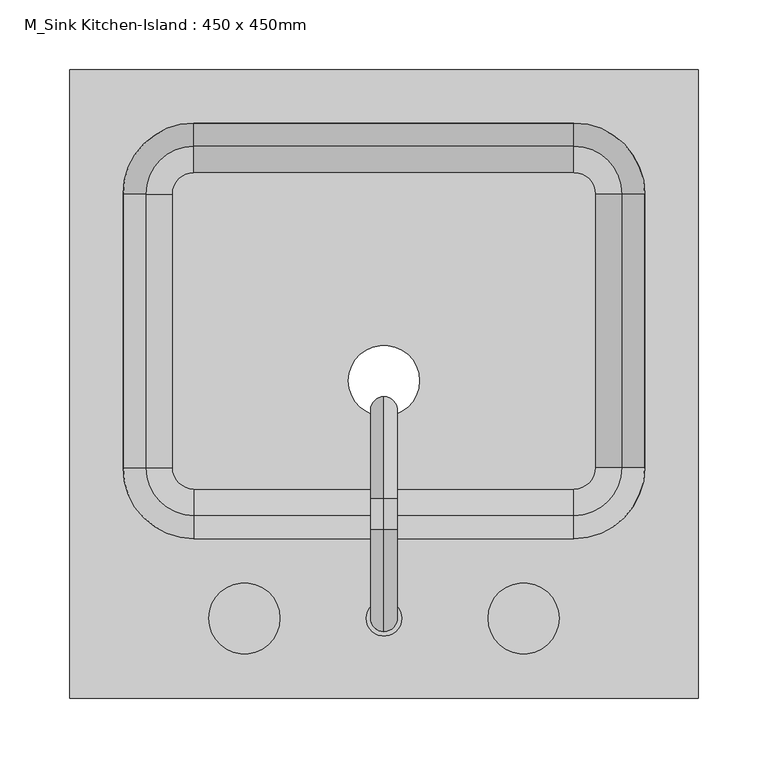
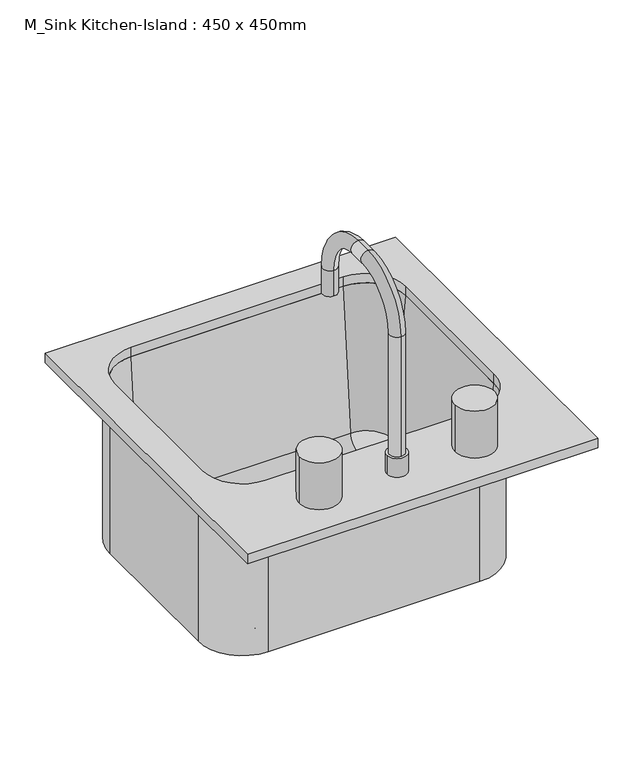
"""IFC4 building model written with IfcOpenShell, lengths in millimetres: flow terminal geometry, M_Sink Kitchen-Island : 450 x 450mm."""

from ifc_helpers import new_model, si_unit, point, frame, frame_2d, origin, place, context, project, spatial, polyline, circle_curve, ellipse_curve, trimmed, segment, composite_curve, outline, extrude, source, transform, mapped, element, save
from ifc_brep_helpers import plane_surface, cylinder_surface, revolved_surface, advanced_brep


def m_sink_kitchen_island_450_x_450mm_f6c2c534(model_context):
    return source(origin(), model_context, "Body", "SolidModel", [
        advanced_brep(
        [(208.9392406, -62.2454011, 684.1), (208.9392406, -62.2454011, 900.0), (151.7892406, -119.3954011, 900.0), (151.7892406, -119.3954011, 684.1), (-120.4107594, -119.3954011, 684.1), (-177.5607594, -62.2454011, 684.1), (-177.5607594, 133.7545989, 684.1), (-120.4107594, 190.9045989, 684.1), (151.7892406, 190.9045989, 684.1), (208.9392406, 133.7545989, 684.1), (-9.7107594, 0.0, 684.1), (41.0892406, 0.0, 684.1), (167.0776588, -62.2454011, 693.625), (167.0776588, 133.7545989, 693.625), (151.7892406, 149.0430171, 693.625), (-120.4107594, 149.0430171, 693.625), (-135.6991776, 133.7545989, 693.625), (-135.6991776, -62.2454011, 693.625), (-120.4107594, -77.5338193, 693.625), (151.7892406, -77.5338193, 693.625), (-9.7107594, 0.0, 693.625), (41.0892406, 0.0, 693.625), (151.7892406, -96.5113283, 711.0146831), (186.0551678, -62.2454011, 711.0146831), (151.7892406, -113.0454011, 900.0), (202.5892406, -62.2454011, 900.0), (208.9392406, 133.7545989, 900.0), (186.0551678, 133.7545989, 711.0146831), (202.5892406, 133.7545989, 900.0), (151.7892406, 190.9045989, 900.0), (151.7892406, 168.0205261, 711.0146831), (151.7892406, 184.5545989, 900.0), (-120.4107594, 190.9045989, 900.0), (-120.4107594, 168.0205261, 711.0146831), (-120.4107594, 184.5545989, 900.0), (-177.5607594, 133.7545989, 900.0), (-154.6766866, 133.7545989, 711.0146831), (-171.2107594, 133.7545989, 900.0), (-177.5607594, -62.2454011, 900.0), (-154.6766866, -62.2454011, 711.0146831), (-171.2107594, -62.2454011, 900.0), (-120.4107594, -119.3954011, 900.0), (-120.4107594, -96.5113283, 711.0146831), (-120.4107594, -113.0454011, 900.0)],
        [
            (0, 1),
            (1, 2, circle_curve(frame((151.7892406, -62.2454011, 900.0), z_axis=(0.0, 0.0, -1.0), x_axis=(0.0, -1.0, 0.0)), 57.15)),
            (2, 3),
            (3, 0, circle_curve(frame((151.7892406, -62.2454011, 684.1), z_axis=(0.0, 0.0, 1.0), x_axis=(0.0, -1.0, 0.0)), 57.15)),
            (3, 4),
            (4, 5, circle_curve(frame((-120.4107594, -62.2454011, 684.1), z_axis=(0.0, 0.0, -1.0), x_axis=(-1.0, 0.0, 0.0)), 57.15)),
            (5, 6),
            (6, 7, circle_curve(frame((-120.4107594, 133.7545989, 684.1), z_axis=(0.0, 0.0, -1.0), x_axis=(0.0, 1.0, 0.0)), 57.15)),
            (7, 8),
            (8, 9, circle_curve(frame((151.7892406, 133.7545989, 684.1), z_axis=(0.0, 0.0, -1.0), x_axis=(1.0, 0.0, 0.0)), 57.15)),
            (9, 0),
            (10, 11, circle_curve(frame((15.6892406, 0.0, 684.1), z_axis=(0.0, 0.0, 1.0), x_axis=(1.0, 0.0, 0.0)), 25.4)),
            (11, 10, circle_curve(frame((15.6892406, 0.0, 684.1), z_axis=(0.0, 0.0, 1.0), x_axis=(1.0, 0.0, 0.0)), 25.4)),
            (12, 13),
            (13, 14, circle_curve(frame((151.7892406, 133.7545989, 693.625), z_axis=(0.0, 0.0, 1.0), x_axis=(1.0, 0.0, 0.0)), 15.2884182)),
            (14, 15),
            (15, 16, circle_curve(frame((-120.4107594, 133.7545989, 693.625), z_axis=(0.0, 0.0, 1.0), x_axis=(0.0, 1.0, 0.0)), 15.2884182)),
            (16, 17),
            (17, 18, circle_curve(frame((-120.4107594, -62.2454011, 693.625), z_axis=(0.0, 0.0, 1.0), x_axis=(-1.0, 0.0, 0.0)), 15.2884182)),
            (18, 19),
            (19, 12, circle_curve(frame((151.7892406, -62.2454011, 693.625), z_axis=(0.0, 0.0, 1.0), x_axis=(0.0, -1.0, 0.0)), 15.2884182)),
            (20, 21, circle_curve(frame((15.6892406, 0.0, 693.625), z_axis=(0.0, 0.0, -1.0), x_axis=(1.0, 0.0, 0.0)), 25.4)),
            (21, 20, circle_curve(frame((15.6892406, 0.0, 693.625), z_axis=(0.0, 0.0, -1.0), x_axis=(1.0, 0.0, 0.0)), 25.4)),
            (19, 22, circle_curve(frame((151.7892406, -77.5338193, 712.675), z_axis=(-1.0, 0.0, 0.0), x_axis=(0.0, -1.0, 0.0)), 19.05)),
            (22, 23, circle_curve(frame((151.7892406, -62.2454011, 711.0146831), z_axis=(0.0, 0.0, 1.0), x_axis=(0.0, -1.0, 0.0)), 34.2659272)),
            (23, 12, circle_curve(frame((167.0776588, -62.2454011, 712.675), z_axis=(0.0, 1.0, 0.0), x_axis=(1.0, 0.0, 0.0)), 19.05)),
            (22, 24),
            (24, 25, circle_curve(frame((151.7892406, -62.2454011, 900.0), z_axis=(0.0, 0.0, 1.0), x_axis=(0.0, -1.0, 0.0)), 50.8)),
            (25, 23),
            (1, 25),
            (24, 2),
            (9, 26),
            (26, 1),
            (23, 27),
            (27, 13, circle_curve(frame((167.0776588, 133.7545989, 712.675), z_axis=(0.0, 1.0, 0.0), x_axis=(1.0, 0.0, 0.0)), 19.05)),
            (25, 28),
            (28, 27),
            (26, 28),
            (8, 29),
            (29, 26, circle_curve(frame((151.7892406, 133.7545989, 900.0), z_axis=(0.0, 0.0, -1.0), x_axis=(1.0, 0.0, 0.0)), 57.15)),
            (27, 30, circle_curve(frame((151.7892406, 133.7545989, 711.0146831), z_axis=(0.0, 0.0, 1.0), x_axis=(1.0, 0.0, 0.0)), 34.2659272)),
            (30, 14, circle_curve(frame((151.7892406, 149.0430171, 712.675), z_axis=(-1.0, 0.0, 0.0), x_axis=(0.0, 1.0, 0.0)), 19.05)),
            (28, 31, circle_curve(frame((151.7892406, 133.7545989, 900.0), z_axis=(0.0, 0.0, 1.0), x_axis=(1.0, 0.0, 0.0)), 50.8)),
            (31, 30),
            (29, 31),
            (7, 32),
            (32, 29),
            (30, 33),
            (33, 15, circle_curve(frame((-120.4107594, 149.0430171, 712.675), z_axis=(-1.0, 0.0, 0.0), x_axis=(0.0, 1.0, 0.0)), 19.05)),
            (31, 34),
            (34, 33),
            (32, 34),
            (6, 35),
            (35, 32, circle_curve(frame((-120.4107594, 133.7545989, 900.0), z_axis=(0.0, 0.0, -1.0), x_axis=(0.0, 1.0, 0.0)), 57.15)),
            (33, 36, circle_curve(frame((-120.4107594, 133.7545989, 711.0146831), z_axis=(0.0, 0.0, 1.0), x_axis=(0.0, 1.0, 0.0)), 34.2659272)),
            (36, 16, circle_curve(frame((-135.6991776, 133.7545989, 712.675), z_axis=(0.0, -1.0, 0.0), x_axis=(-1.0, 0.0, 0.0)), 19.05)),
            (34, 37, circle_curve(frame((-120.4107594, 133.7545989, 900.0), z_axis=(0.0, 0.0, 1.0), x_axis=(0.0, 1.0, 0.0)), 50.8)),
            (37, 36),
            (35, 37),
            (5, 38),
            (38, 35),
            (36, 39),
            (39, 17, circle_curve(frame((-135.6991776, -62.2454011, 712.675), z_axis=(0.0, -1.0, 0.0), x_axis=(-1.0, 0.0, 0.0)), 19.05)),
            (37, 40),
            (40, 39),
            (38, 40),
            (4, 41),
            (41, 38, circle_curve(frame((-120.4107594, -62.2454011, 900.0), z_axis=(0.0, 0.0, -1.0), x_axis=(-1.0, 0.0, 0.0)), 57.15)),
            (39, 42, circle_curve(frame((-120.4107594, -62.2454011, 711.0146831), z_axis=(0.0, 0.0, 1.0), x_axis=(-1.0, 0.0, 0.0)), 34.2659272)),
            (42, 18, circle_curve(frame((-120.4107594, -77.5338193, 712.675), z_axis=(1.0, 0.0, 0.0), x_axis=(0.0, -1.0, 0.0)), 19.05)),
            (40, 43, circle_curve(frame((-120.4107594, -62.2454011, 900.0), z_axis=(0.0, 0.0, 1.0), x_axis=(-1.0, 0.0, 0.0)), 50.8)),
            (43, 42),
            (41, 43),
            (2, 41),
            (42, 22),
            (43, 24),
            (21, 11),
            (10, 20),
        ],
        [
            cylinder_surface(frame((151.7892406, -62.2454011, 0.0), z_axis=(0.0, 0.0, -1.0), x_axis=(0.0, -1.0, 0.0)), 57.15),
            plane_surface(frame((151.7892406, -62.2454011, 684.1), z_axis=(0.0, 0.0, -1.0), x_axis=(0.0, -1.0, 0.0))),
            plane_surface(frame((151.7892406, -62.2454011, 693.625), z_axis=(0.0, 0.0, 1.0), x_axis=(0.0, -1.0, 0.0))),
            revolved_surface(trimmed(ellipse_curve(frame((151.7892406, -77.5338193, 712.675), z_axis=(-1.0, 0.0, 0.0), x_axis=(0.0, -1.0, 0.0)), 19.05, 19.05), [point((151.7892406, -77.5338193, 693.625))], [point((151.7892406, -96.5113283, 711.0146831))], True, "CARTESIAN"), (151.7892406, -62.2454011, 0.0), (0.0, 0.0, -1.0)),
            revolved_surface(polyline([(151.7892406, -96.5113283, 711.0146831), (151.7892406, -113.0454011, 900.0)]), (151.7892406, -62.2454011, 0.0), (0.0, 0.0, -1.0)),
            plane_surface(frame((151.7892406, -62.2454011, 900.0), z_axis=(0.0, 0.0, 1.0), x_axis=(0.0, -1.0, 0.0))),
            plane_surface(frame((208.9392406, -62.2454011, 900.0), z_axis=(1.0, 0.0, 0.0), x_axis=(0.0, 1.0, 0.0))),
            revolved_surface(polyline([(186.1276588, 133.7545989, 712.675), (186.1276588, -62.2454011, 712.675)]), (167.0776588, -62.2454011, 712.675), (0.0, 1.0, 0.0)),
            plane_surface(frame((186.0551678, -62.2454011, 711.0146831), z_axis=(-0.9961946980917444, 0.0, 0.0871557427476718), x_axis=(0.0, 1.0, 0.0))),
            plane_surface(frame((202.5892406, -62.2454011, 900.0), z_axis=(0.0, 0.0, 1.0), x_axis=(0.0, 1.0, 0.0))),
            cylinder_surface(frame((151.7892406, 133.7545989, 0.0), z_axis=(0.0, 0.0, -1.0), x_axis=(1.0, 0.0, 0.0)), 57.15),
            revolved_surface(trimmed(ellipse_curve(frame((167.0776588, 133.7545989, 712.675), z_axis=(0.0, -1.0, 0.0), x_axis=(1.0, 0.0, 0.0)), 19.05, 19.05), [point((167.0776588, 133.7545989, 693.625))], [point((186.0551678, 133.7545989, 711.0146831))], True, "CARTESIAN"), (151.7892406, 133.7545989, 0.0), (0.0, 0.0, -1.0)),
            revolved_surface(polyline([(186.0551678, 133.7545989, 711.0146831), (202.5892406, 133.7545989, 900.0)]), (151.7892406, 133.7545989, 0.0), (0.0, 0.0, -1.0)),
            plane_surface(frame((151.7892406, 133.7545989, 900.0), z_axis=(0.0, 0.0, 1.0), x_axis=(1.0, 0.0, 0.0))),
            plane_surface(frame((151.7892406, 190.9045989, 900.0), z_axis=(0.0, 1.0, 0.0), x_axis=(-1.0, 0.0, 0.0))),
            revolved_surface(polyline([(-120.41075939999999, 168.0930171, 712.675), (151.7892406, 168.0930171, 712.675)]), (151.7892406, 149.0430171, 712.675), (-1.0, 0.0, 0.0)),
            plane_surface(frame((151.7892406, 168.0205261, 711.0146831), z_axis=(0.0, -0.9961946980917444, 0.0871557427476718), x_axis=(-1.0, 0.0, 0.0))),
            plane_surface(frame((151.7892406, 184.5545989, 900.0), z_axis=(0.0, 0.0, 1.0), x_axis=(-1.0, 0.0, 0.0))),
            cylinder_surface(frame((-120.4107594, 133.7545989, 0.0), z_axis=(0.0, 0.0, -1.0), x_axis=(0.0, 1.0, 0.0)), 57.15),
            revolved_surface(trimmed(ellipse_curve(frame((-120.4107594, 149.0430171, 712.675), z_axis=(1.0, 0.0, 0.0), x_axis=(0.0, 1.0, 0.0)), 19.05, 19.05), [point((-120.4107594, 149.0430171, 693.625))], [point((-120.4107594, 168.0205261, 711.0146831))], True, "CARTESIAN"), (-120.4107594, 133.7545989, 0.0), (0.0, 0.0, -1.0)),
            revolved_surface(polyline([(-120.4107594, 168.0205261, 711.0146831), (-120.4107594, 184.5545989, 900.0)]), (-120.4107594, 133.7545989, 0.0), (0.0, 0.0, -1.0)),
            plane_surface(frame((-120.4107594, 133.7545989, 900.0), z_axis=(0.0, 0.0, 1.0), x_axis=(0.0, 1.0, 0.0))),
            plane_surface(frame((-177.5607594, 133.7545989, 900.0), z_axis=(-1.0, 0.0, 0.0), x_axis=(0.0, -1.0, 0.0))),
            revolved_surface(polyline([(-154.74917760000002, -62.24540110000001, 712.675), (-154.74917760000002, 133.7545989, 712.675)]), (-135.6991776, 133.7545989, 712.675), (0.0, -1.0, 0.0)),
            plane_surface(frame((-154.6766866, 133.7545989, 711.0146831), z_axis=(0.9961946980917444, 0.0, 0.0871557427476718), x_axis=(0.0, -1.0, 0.0))),
            plane_surface(frame((-171.2107594, 133.7545989, 900.0), z_axis=(0.0, 0.0, 1.0), x_axis=(0.0, -1.0, 0.0))),
            cylinder_surface(frame((-120.4107594, -62.2454011, 0.0), z_axis=(0.0, 0.0, -1.0), x_axis=(-1.0, 0.0, 0.0)), 57.15),
            revolved_surface(trimmed(ellipse_curve(frame((-135.6991776, -62.2454011, 712.675), z_axis=(0.0, 1.0, 0.0), x_axis=(-1.0, 0.0, 0.0)), 19.05, 19.05), [point((-135.6991776, -62.2454011, 693.625))], [point((-154.6766866, -62.2454011, 711.0146831))], True, "CARTESIAN"), (-120.4107594, -62.2454011, 0.0), (0.0, 0.0, -1.0)),
            revolved_surface(polyline([(-154.6766866, -62.2454011, 711.0146831), (-171.2107594, -62.2454011, 900.0)]), (-120.4107594, -62.2454011, 0.0), (0.0, 0.0, -1.0)),
            plane_surface(frame((-120.4107594, -62.2454011, 900.0), z_axis=(0.0, 0.0, 1.0), x_axis=(-1.0, 0.0, 0.0))),
            plane_surface(frame((-120.4107594, -119.3954011, 900.0), z_axis=(0.0, -1.0, 0.0), x_axis=(1.0, 0.0, 0.0))),
            revolved_surface(polyline([(151.78924059999997, -96.5838193, 712.675), (-120.4107594, -96.5838193, 712.675)]), (-120.4107594, -77.5338193, 712.675), (1.0, 0.0, 0.0)),
            plane_surface(frame((-120.4107594, -96.5113283, 711.0146831), z_axis=(0.0, 0.9961946980917444, 0.0871557427476718), x_axis=(1.0, 0.0, 0.0))),
            plane_surface(frame((-120.4107594, -113.0454011, 900.0), z_axis=(0.0, 0.0, 1.0), x_axis=(1.0, 0.0, 0.0))),
            revolved_surface(polyline([(41.0892406, 0.0, 684.1), (41.0892406, 0.0, 693.625)]), (15.6892406, 0.0, 0.0), (0.0, 0.0, -1.0)),
        ],
        [
            (0, [[1, 2, 3, 4]]),
            (1, [[5, 6, 7, 8, 9, 10, 11, -4], [12, 13]]),
            (2, [[14, 15, 16, 17, 18, 19, 20, 21], [22, 23]]),
            (3, [[24, 25, 26, -21]]),
            (4, [[27, 28, 29, -25]]),
            (5, [[30, -28, 31, -2]]),
            (6, [[-11, 32, 33, -1]]),
            (7, [[34, 35, -14, -26]]),
            (8, [[36, 37, -34, -29]]),
            (9, [[-33, 38, -36, -30]]),
            (10, [[-10, 39, 40, -32]]),
            (11, [[41, 42, -15, -35]]),
            (12, [[43, 44, -41, -37]]),
            (13, [[-40, 45, -43, -38]]),
            (14, [[-9, 46, 47, -39]]),
            (15, [[48, 49, -16, -42]]),
            (16, [[50, 51, -48, -44]]),
            (17, [[-47, 52, -50, -45]]),
            (18, [[-8, 53, 54, -46]]),
            (19, [[55, 56, -17, -49]]),
            (20, [[57, 58, -55, -51]]),
            (21, [[-54, 59, -57, -52]]),
            (22, [[-7, 60, 61, -53]]),
            (23, [[62, 63, -18, -56]]),
            (24, [[64, 65, -62, -58]]),
            (25, [[-61, 66, -64, -59]]),
            (26, [[-6, 67, 68, -60]]),
            (27, [[69, 70, -19, -63]]),
            (28, [[71, 72, -69, -65]]),
            (29, [[-68, 73, -71, -66]]),
            (30, [[74, -67, -5, -3]]),
            (31, [[-20, -70, 75, -24]]),
            (32, [[-75, -72, 76, -27]]),
            (33, [[-76, -73, -74, -31]]),
            (34, [[77, -12, 78, -23]]),
            (34, [[-78, -13, -77, -22]]),
        ],
    ),
        advanced_brep(
        [(2.9892406, -170.1954011, 912.7), (28.3892406, -170.1954011, 912.7), (15.6892406, -179.7204011, 1100.025), (15.6892406, -179.7204011, 938.1), (15.6892406, -160.6704011, 938.1), (15.6892406, -160.6704011, 1100.025), (15.6892406, -106.6954011, 1154.0), (15.6892406, -106.6954011, 1173.05), (15.6892406, -84.4704011, 1154.0), (15.6892406, -84.4704011, 1173.05), (15.6892406, -30.4954011, 1100.025), (15.6892406, -11.4454011, 1100.025), (15.6892406, -11.4454011, 1065.1), (15.6892406, -30.4954011, 1065.1), (2.9892406, -170.1954011, 938.1), (28.3892406, -170.1954011, 938.1)],
        [
            (0, 1, circle_curve(frame((15.6892406, -170.1954011, 912.7), z_axis=(0.0, 0.0, -1.0), x_axis=(1.0, 0.0, 0.0)), 12.7)),
            (1, 0, circle_curve(frame((15.6892406, -170.1954011, 912.7), z_axis=(0.0, 0.0, -1.0), x_axis=(1.0, 0.0, 0.0)), 12.7)),
            (2, 3),
            (3, 4, circle_curve(frame((15.6892406, -170.1954011, 938.1), z_axis=(0.0, 0.0, 1.0), x_axis=(0.0, 1.0, 0.0)), 9.525)),
            (4, 5),
            (5, 2, circle_curve(frame((15.6892406, -170.1954011, 1100.025), z_axis=(0.0, 0.0, -1.0), x_axis=(0.0, 1.0, 0.0)), 9.525)),
            (4, 3, circle_curve(frame((15.6892406, -170.1954011, 938.1), z_axis=(0.0, 0.0, 1.0), x_axis=(0.0, 1.0, 0.0)), 9.525)),
            (2, 5, circle_curve(frame((15.6892406, -170.1954011, 1100.025), z_axis=(0.0, 0.0, -1.0), x_axis=(0.0, 1.0, 0.0)), 9.525)),
            (5, 6, circle_curve(frame((15.6892406, -106.6954011, 1100.025), z_axis=(-1.0, 0.0, 0.0), x_axis=(0.0, -1.0, 0.0)), 53.975)),
            (6, 7, circle_curve(frame((15.6892406, -106.6954011, 1163.525), z_axis=(0.0, -1.0, 0.0), x_axis=(0.0, 0.0, -1.0)), 9.525)),
            (7, 2, circle_curve(frame((15.6892406, -106.6954011, 1100.025), z_axis=(1.0, 0.0, 0.0), x_axis=(0.0, -1.0, 0.0)), 73.025)),
            (7, 6, circle_curve(frame((15.6892406, -106.6954011, 1163.525), z_axis=(0.0, -1.0, 0.0), x_axis=(0.0, 0.0, -1.0)), 9.525)),
            (6, 8),
            (8, 9, circle_curve(frame((15.6892406, -84.4704011, 1163.525), z_axis=(0.0, -1.0, 0.0), x_axis=(0.0, 0.0, -1.0)), 9.525)),
            (9, 7),
            (9, 8, circle_curve(frame((15.6892406, -84.4704011, 1163.525), z_axis=(0.0, -1.0, 0.0), x_axis=(0.0, 0.0, -1.0)), 9.525)),
            (8, 10, circle_curve(frame((15.6892406, -84.4704011, 1100.025), z_axis=(-1.0, 0.0, 0.0), x_axis=(0.0, 0.0, 1.0)), 53.975)),
            (10, 11, circle_curve(frame((15.6892406, -20.9704011, 1100.025), z_axis=(0.0, 0.0, 1.0), x_axis=(0.0, -1.0, 0.0)), 9.525)),
            (11, 9, circle_curve(frame((15.6892406, -84.4704011, 1100.025), z_axis=(1.0, 0.0, 0.0), x_axis=(0.0, 0.0, 1.0)), 73.025)),
            (11, 10, circle_curve(frame((15.6892406, -20.9704011, 1100.025), z_axis=(0.0, 0.0, 1.0), x_axis=(0.0, -1.0, 0.0)), 9.525)),
            (12, 13, circle_curve(frame((15.6892406, -20.9704011, 1065.1), z_axis=(0.0, 0.0, -1.0), x_axis=(0.0, -1.0, 0.0)), 9.525)),
            (13, 12, circle_curve(frame((15.6892406, -20.9704011, 1065.1), z_axis=(0.0, 0.0, -1.0), x_axis=(0.0, -1.0, 0.0)), 9.525)),
            (10, 13),
            (12, 11),
            (14, 15, circle_curve(frame((15.6892406, -170.1954011, 938.1), z_axis=(0.0, 0.0, 1.0), x_axis=(1.0, 0.0, 0.0)), 12.7)),
            (15, 14, circle_curve(frame((15.6892406, -170.1954011, 938.1), z_axis=(0.0, 0.0, 1.0), x_axis=(1.0, 0.0, 0.0)), 12.7)),
            (15, 1),
            (0, 14),
        ],
        [
            plane_surface(frame((15.6892406, -160.6704011, 912.7), z_axis=(0.0, 0.0, -1.0), x_axis=(1.0, 0.0, 0.0))),
            cylinder_surface(frame((15.6892406, -170.1954011, 912.7), z_axis=(0.0, 0.0, -1.0), x_axis=(0.0, 1.0, 0.0)), 9.525),
            revolved_surface(trimmed(ellipse_curve(frame((15.6892406, -170.1954011, 1100.025), z_axis=(0.0, 0.0, 1.0), x_axis=(0.0, 1.0, 0.0)), 9.525, 9.525), [point((15.6892406, -179.7204011, 1100.025))], [point((15.6892406, -160.6704011, 1100.025))], True, "CARTESIAN"), (15.6892406, -106.6954011, 1100.025), (1.0, 0.0, 0.0)),
            revolved_surface(trimmed(ellipse_curve(frame((15.6892406, -170.1954011, 1100.025), z_axis=(0.0, 0.0, 1.0), x_axis=(0.0, 1.0, 0.0)), 9.525, 9.525), [point((15.6892406, -160.6704011, 1100.025))], [point((15.6892406, -179.7204011, 1100.025))], True, "CARTESIAN"), (15.6892406, -106.6954011, 1100.025), (1.0, 0.0, 0.0)),
            cylinder_surface(frame((15.6892406, -106.6954011, 1163.525), z_axis=(0.0, -1.0, 0.0), x_axis=(0.0, 0.0, -1.0)), 9.525),
            revolved_surface(trimmed(ellipse_curve(frame((15.6892406, -84.4704011, 1163.525), z_axis=(0.0, 1.0, 0.0), x_axis=(0.0, 0.0, -1.0)), 9.525, 9.525), [point((15.6892406, -84.4704011, 1173.05))], [point((15.6892406, -84.4704011, 1154.0))], True, "CARTESIAN"), (15.6892406, -84.4704011, 1100.025), (1.0, 0.0, 0.0)),
            revolved_surface(trimmed(ellipse_curve(frame((15.6892406, -84.4704011, 1163.525), z_axis=(0.0, 1.0, 0.0), x_axis=(0.0, 0.0, -1.0)), 9.525, 9.525), [point((15.6892406, -84.4704011, 1154.0))], [point((15.6892406, -84.4704011, 1173.05))], True, "CARTESIAN"), (15.6892406, -84.4704011, 1100.025), (1.0, 0.0, 0.0)),
            plane_surface(frame((15.6892406, -11.4454011, 1065.1), z_axis=(0.0, 0.0, -1.0), x_axis=(-1.0, 0.0, 0.0))),
            cylinder_surface(frame((15.6892406, -20.9704011, 1100.025), z_axis=(0.0, 0.0, 1.0), x_axis=(0.0, -1.0, 0.0)), 9.525),
            plane_surface(frame((28.3892406, -170.1954011, 938.1), z_axis=(0.0, 0.0, 1.0), x_axis=(0.0, -1.0, 0.0))),
            cylinder_surface(frame((15.6892406, -170.1954011, 912.7), z_axis=(0.0, 0.0, 1.0), x_axis=(1.0, 0.0, 0.0)), 12.7),
        ],
        [
            (0, [[1, 2]]),
            (1, [[3, 4, 5, 6]]),
            (1, [[-5, 7, -3, 8]]),
            (2, [[9, 10, 11, -6]]),
            (3, [[-11, 12, -9, -8]]),
            (4, [[13, 14, 15, -10]]),
            (4, [[-15, 16, -13, -12]]),
            (5, [[17, 18, 19, -14]]),
            (6, [[-19, 20, -17, -16]]),
            (7, [[21, 22]]),
            (8, [[23, -21, 24, -18]]),
            (8, [[-24, -22, -23, -20]]),
            (9, [[25, 26], [-7, -4]]),
            (10, [[27, -1, 28, -26]]),
            (10, [[-28, -2, -27, -25]]),
        ],
    ),
        extrude(outline(composite_curve([segment(trimmed(circle_curve(frame_2d((-84.3107594, -170.1954011)), 25.4), [point((-109.7107594, -170.1954011))], [point((-58.9107594, -170.1954011))], False, "CARTESIAN"), True, "CONTINUOUS"), segment(trimmed(circle_curve(frame_2d((-84.3107594, -170.1954011)), 25.4), [point((-58.9107594, -170.1954011))], [point((-109.7107594, -170.1954011))], False, "CARTESIAN"), True, "CONTINUOUS")], self_intersect=False)), frame((0.0, 0.0, 912.7), z_axis=(0.0, 0.0, 1.0), x_axis=(1.0, 0.0, 0.0)), (0.0, 0.0, 1.0), 63.5),
        extrude(outline(composite_curve([segment(trimmed(circle_curve(frame_2d((115.6892406, -170.1954011)), 25.4), [point((90.2892406, -170.1954011))], [point((141.0892406, -170.1954011))], False, "CARTESIAN"), True, "CONTINUOUS"), segment(trimmed(circle_curve(frame_2d((115.6892406, -170.1954011)), 25.4), [point((141.0892406, -170.1954011))], [point((90.2892406, -170.1954011))], False, "CARTESIAN"), True, "CONTINUOUS")], self_intersect=False)), frame((0.0, 0.0, 912.7), z_axis=(0.0, 0.0, 1.0), x_axis=(1.0, 0.0, 0.0)), (0.0, 0.0, 1.0), 63.5),
        extrude(outline(polyline([(240.6892406, -227.3454011), (-209.3107594, -227.3454011), (-209.3107594, 222.6545989), (240.6892406, 222.6545989), (240.6892406, -227.3454011)]), holes=[composite_curve([segment(trimmed(circle_curve(frame_2d((151.7892406, -62.2454011)), 50.8), [point((151.7892406, -113.0454011))], [point((202.5892406, -62.2454011))], True, "CARTESIAN"), True, "CONTINUOUS"), segment(polyline([(202.5892406, -62.2454011), (202.5892406, 133.7545989)]), True, "CONTINUOUS"), segment(trimmed(circle_curve(frame_2d((151.7892406, 133.7545989)), 50.8), [point((202.5892406, 133.7545989))], [point((151.7892406, 184.5545989))], True, "CARTESIAN"), True, "CONTINUOUS"), segment(polyline([(151.7892406, 184.5545989), (-120.4107594, 184.5545989)]), True, "CONTINUOUS"), segment(trimmed(circle_curve(frame_2d((-120.4107594, 133.7545989)), 50.8), [point((-120.4107594, 184.5545989))], [point((-171.2107594, 133.7545989))], True, "CARTESIAN"), True, "CONTINUOUS"), segment(polyline([(-171.2107594, 133.7545989), (-171.2107594, -62.2454011)]), True, "CONTINUOUS"), segment(trimmed(circle_curve(frame_2d((-120.4107594, -62.2454011)), 50.8), [point((-171.2107594, -62.2454011))], [point((-120.4107594, -113.0454011))], True, "CARTESIAN"), True, "CONTINUOUS"), segment(polyline([(-120.4107594, -113.0454011), (151.7892406, -113.0454011)]), True, "CONTINUOUS")], self_intersect=False)]), frame((0.0, 0.0, 900.0), z_axis=(0.0, 0.0, 1.0), x_axis=(1.0, 0.0, 0.0)), (0.0, 0.0, 1.0), 12.7),
    ])


if __name__ == "__main__":
    model = new_model("IFC4")
    model_context = context("Model", 3, world=origin())
    ifc_project = project(units=[si_unit("LENGTHUNIT", "METRE", prefix="MILLI")], contexts=[model_context])
    site = spatial("IfcSite", under=ifc_project)
    building = spatial("IfcBuilding", under=site)
    placement = place(None, origin())
    m_sink_kitchen_island_450_x_450mm_shape = m_sink_kitchen_island_450_x_450mm_f6c2c534(model_context)
    element("IfcFlowTerminal", 1, ObjectType="M_Sink Kitchen-Island : 450 x 450mm", at=placement, inside=building, context=model_context, shape_type="MappedRepresentation", body=[
        mapped(m_sink_kitchen_island_450_x_450mm_shape, transform((0.0, 0.0, 0.0), x_axis=(1.0, 0.0, 0.0), y_axis=(0.0, 1.0, 0.0), z_axis=(0.0, 0.0, 1.0))),
    ])
    save(model, "model.ifc")

# Revit data of these elements
# Type "M_Sink Kitchen-Island : 450 x 450mm"
#   Counter Height [instance default] = 2.952756 ft
#   Depth = 1.476378 ft
#   Width = 1.476378 ft
#   Fixture Material = Steel, Polished
#   Sink Material = Steel, Polished
#   Default Elevation = 0
# Element 1 (IfcFlowTerminal, "M_Sink Kitchen-Island : 450 x 450mm")
#   Materials on its faces: "Steel, Polished"
# Materials
#   "Steel, Polished": class "Metal", colour RGB 57 57 57, transparency 0, Description = "Polished steel", Cost = 0
